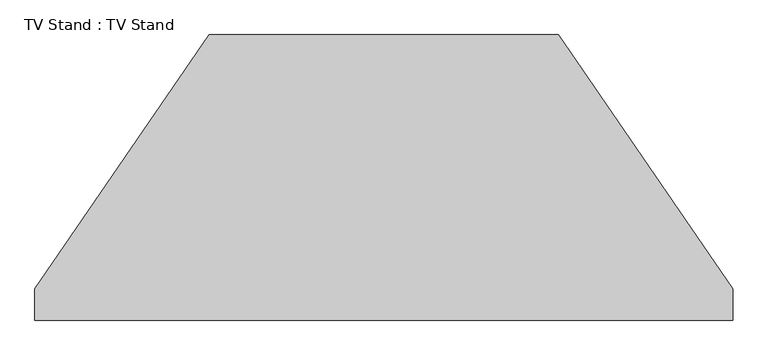
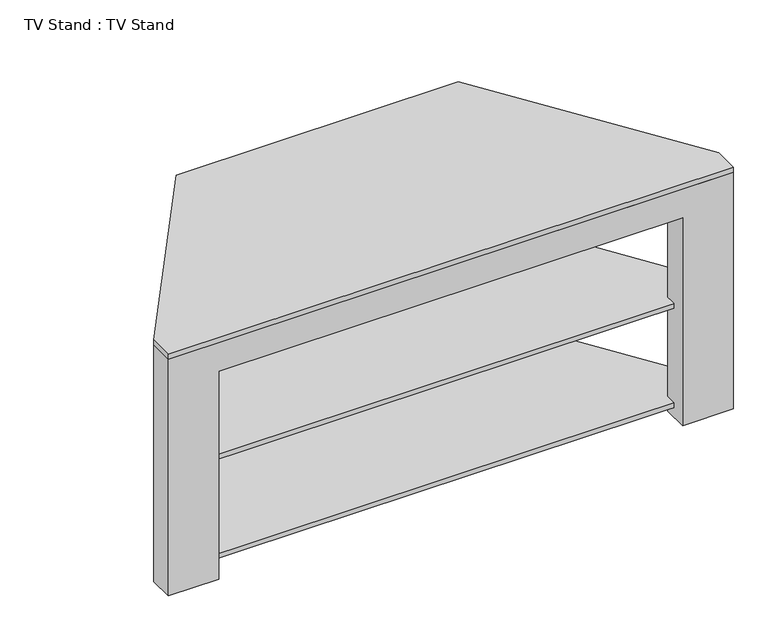
"""IFC4 building model written with IfcOpenShell, lengths in millimetres: furniture geometry, TV Stand : TV Stand."""

from ifc_helpers import new_model, si_unit, point, frame, frame_2d, origin, place, context, project, spatial, polyline, circle_curve, trimmed, segment, composite_curve, outline, extrude, faceted_brep, source, transform, mapped, element, save


def tv_stand_tv_stand_6ce107e5(model_context):
    return source(origin(), model_context, "Body", "SolidModel", [
        extrude(outline(polyline([(425.1724814, -30.0), (633.9880021, -334.3295634), (633.9880021, -427.2), (-383.6119979, -427.2), (-383.6119979, -334.3295634), (-174.7964773, -30.0), (425.1724814, -30.0)])), frame((0.0, 0.0, 20.0), z_axis=(0.0, 0.0, 1.0), x_axis=(1.0, 0.0, 0.0)), (0.0, 0.0, 1.0), 10.0),
        extrude(outline(polyline([(425.1724814, -30.0), (633.9880021, -334.3295634), (633.9880021, -427.2), (-383.6119979, -427.2), (-383.6119979, -334.3295634), (-174.7964773, -30.0), (425.1724814, -30.0)])), frame((0.0, 0.0, 227.65), z_axis=(0.0, 0.0, 1.0), x_axis=(1.0, 0.0, 0.0)), (0.0, 0.0, 1.0), 10.0),
        extrude(outline(polyline([(404.5880021, 0.0), (683.9880021, -407.2), (683.9880021, -457.2), (-433.6119979, -457.2), (-433.6119979, -407.2), (-154.2119979, 0.0), (404.5880021, 0.0)])), frame((0.0, 0.0, 495.3), z_axis=(0.0, 0.0, 1.0), x_axis=(1.0, 0.0, 0.0)), (0.0, 0.0, 1.0), 10.0),
        extrude(outline(polyline([(-50.0, 495.3), (0.0, 495.3), (0.0, 0.0), (-50.0, 0.0), (-50.0, 20.0), (-30.0, 20.0), (-30.0, 30.0), (-50.0, 30.0), (-50.0, 227.65), (-30.0, 227.65), (-30.0, 237.65), (-50.0, 237.65), (-50.0, 495.3)])), frame((-154.2119979, 0.0, 0.0), z_axis=(1.0, 0.0, 0.0), x_axis=(0.0, 1.0, 0.0)), (0.0, 0.0, 1.0), 100.0),
        extrude(outline(polyline([(-50.0, 495.3), (0.0, 495.3), (0.0, 0.0), (-50.0, 0.0), (-50.0, 20.0), (-30.0, 20.0), (-30.0, 30.0), (-50.0, 30.0), (-50.0, 227.65), (-30.0, 227.65), (-30.0, 237.65), (-50.0, 237.65), (-50.0, 495.3)])), frame((304.5880021, 0.0, 0.0), z_axis=(1.0, 0.0, 0.0), x_axis=(0.0, 1.0, 0.0)), (0.0, 0.0, 1.0), 100.0),
        faceted_brep([(-433.6119979, -457.2, 0.0), (-333.6119979, -457.2, 0.0), (-333.6119979, -457.2, 435.3), (583.9880021, -457.2, 435.3), (583.9880021, -457.2, 0.0), (683.9880021, -457.2, 0.0), (683.9880021, -457.2, 495.3), (-433.6119979, -457.2, 495.3), (-433.6119979, -407.2, 0.0), (-433.6119979, -407.2, 495.3), (683.9880021, -407.2, 495.3), (683.9880021, -407.2, 0.0), (583.9880021, -407.2, 0.0), (583.9880021, -407.2, 20.0), (633.9880021, -407.2, 20.0), (633.9880021, -407.2, 30.0), (583.9880021, -407.2, 30.0), (583.9880021, -407.2, 227.65), (633.9880021, -407.2, 227.65), (633.9880021, -407.2, 237.65), (583.9880021, -407.2, 237.65), (583.9880021, -407.2, 435.3), (-333.6119979, -407.2, 435.3), (-333.6119979, -407.2, 237.65), (-383.6119979, -407.2, 237.65), (-383.6119979, -407.2, 227.65), (-333.6119979, -407.2, 227.65), (-333.6119979, -407.2, 30.0), (-383.6119979, -407.2, 30.0), (-383.6119979, -407.2, 20.0), (-333.6119979, -407.2, 20.0), (-333.6119979, -407.2, 0.0), (-333.6119979, -427.2, 20.0), (-333.6119979, -427.2, 30.0), (-333.6119979, -427.2, 227.65), (-333.6119979, -427.2, 237.65), (583.9880021, -427.2, 237.65), (583.9880021, -427.2, 227.65), (583.9880021, -427.2, 30.0), (583.9880021, -427.2, 20.0), (633.9880021, -427.2, 237.65), (-383.6119979, -427.2, 237.65), (-383.6119979, -427.2, 227.65), (633.9880021, -427.2, 227.65), (633.9880021, -427.2, 30.0), (-383.6119979, -427.2, 30.0), (-383.6119979, -427.2, 20.0), (633.9880021, -427.2, 20.0)], [[[0, 1, 2, 3, 4, 5, 6, 7]], [[8, 9, 10, 11, 12, 13, 14, 15, 16, 17, 18, 19, 20, 21, 22, 23, 24, 25, 26, 27, 28, 29, 30, 31]], [[1, 0, 8, 31]], [[2, 1, 31, 30, 32, 33, 27, 26, 34, 35, 23, 22]], [[3, 2, 22, 21]], [[4, 3, 21, 20, 36, 37, 17, 16, 38, 39, 13, 12]], [[5, 4, 12, 11]], [[6, 5, 11, 10]], [[7, 6, 10, 9]], [[0, 7, 9, 8]], [[19, 40, 36, 20]], [[35, 41, 24, 23]], [[25, 42, 34, 26]], [[37, 43, 18, 17]], [[41, 42, 25, 24]], [[42, 41, 35, 34]], [[40, 43, 37, 36]], [[43, 40, 19, 18]], [[15, 44, 38, 16]], [[33, 45, 28, 27]], [[29, 46, 32, 30]], [[39, 47, 14, 13]], [[45, 46, 29, 28]], [[46, 45, 33, 32]], [[44, 47, 39, 38]], [[47, 44, 15, 14]]]),
        extrude(outline(polyline([(0.0, 304.5880021), (495.3, 304.5880021), (495.3, -54.2119979), (0.0, -54.2119979), (0.0, 304.5880021)]), holes=[composite_curve([segment(polyline([(242.65, 145.1700818), (242.65, 105.2059224)]), True, "CONTINUOUS"), segment(trimmed(circle_curve(frame_2d((255.15, 105.2059224)), 12.5), [point((242.65, 105.2059224))], [point((267.65, 105.2059224))], True, "CARTESIAN"), True, "CONTINUOUS"), segment(polyline([(267.65, 105.2059224), (267.65, 145.1700818)]), True, "CONTINUOUS"), segment(trimmed(circle_curve(frame_2d((255.15, 145.1700818)), 12.5), [point((267.65, 145.1700818))], [point((242.65, 145.1700818))], True, "CARTESIAN"), True, "CONTINUOUS")], self_intersect=False), composite_curve([segment(polyline([(35.0, 145.1880021), (35.0, 105.2059224)]), True, "CONTINUOUS"), segment(trimmed(circle_curve(frame_2d((47.5, 105.2059224)), 12.5), [point((35.0, 105.2059224))], [point((60.0, 105.2059224))], True, "CARTESIAN"), True, "CONTINUOUS"), segment(polyline([(60.0, 105.2059224), (60.0, 145.1880021)]), True, "CONTINUOUS"), segment(trimmed(circle_curve(frame_2d((47.5, 145.1880021)), 12.5), [point((60.0, 145.1880021))], [point((35.0, 145.1880021))], True, "CARTESIAN"), True, "CONTINUOUS")], self_intersect=False)]), frame((0.0, -30.0, 0.0), z_axis=(0.0, 1.0, 0.0), x_axis=(0.0, 0.0, 1.0)), (0.0, 0.0, 1.0), 10.0),
    ])


if __name__ == "__main__":
    model = new_model("IFC4")
    model_context = context("Model", 3, world=origin())
    ifc_project = project(units=[si_unit("LENGTHUNIT", "METRE", prefix="MILLI")], contexts=[model_context])
    site = spatial("IfcSite", under=ifc_project)
    building = spatial("IfcBuilding", under=site)
    placement = place(None, origin())
    tv_stand_tv_stand_shape = tv_stand_tv_stand_6ce107e5(model_context)
    element("IfcFurniture", 1, ObjectType="TV Stand : TV Stand", at=placement, inside=building, context=model_context, shape_type="MappedRepresentation", body=[
        mapped(tv_stand_tv_stand_shape, transform((0.0, 0.0, 0.0), x_axis=(1.0, 0.0, 0.0), y_axis=(0.0, 1.0, 0.0), z_axis=(0.0, 0.0, 1.0))),
    ])
    save(model, "model.ifc")

# Revit data of these elements
# Type "TV Stand : TV Stand"
#   Depth = 1' - 6"
#   Width = 3' - 8"
#   Height = 1' - 7 1/2"
#   Finish = Melamine - Gray
#   Default Elevation = 0
# Element 1 (IfcFurniture, "TV Stand : TV Stand")
#   Materials on its faces: "Melamine - Gray", "Glass - Shelves"
# Materials
#   "Melamine - Gray": class "Wood", colour RGB 49 49 49, transparency 0
#   "Glass - Shelves": class "Glass", colour RGB 167 167 167, transparency 0.9
